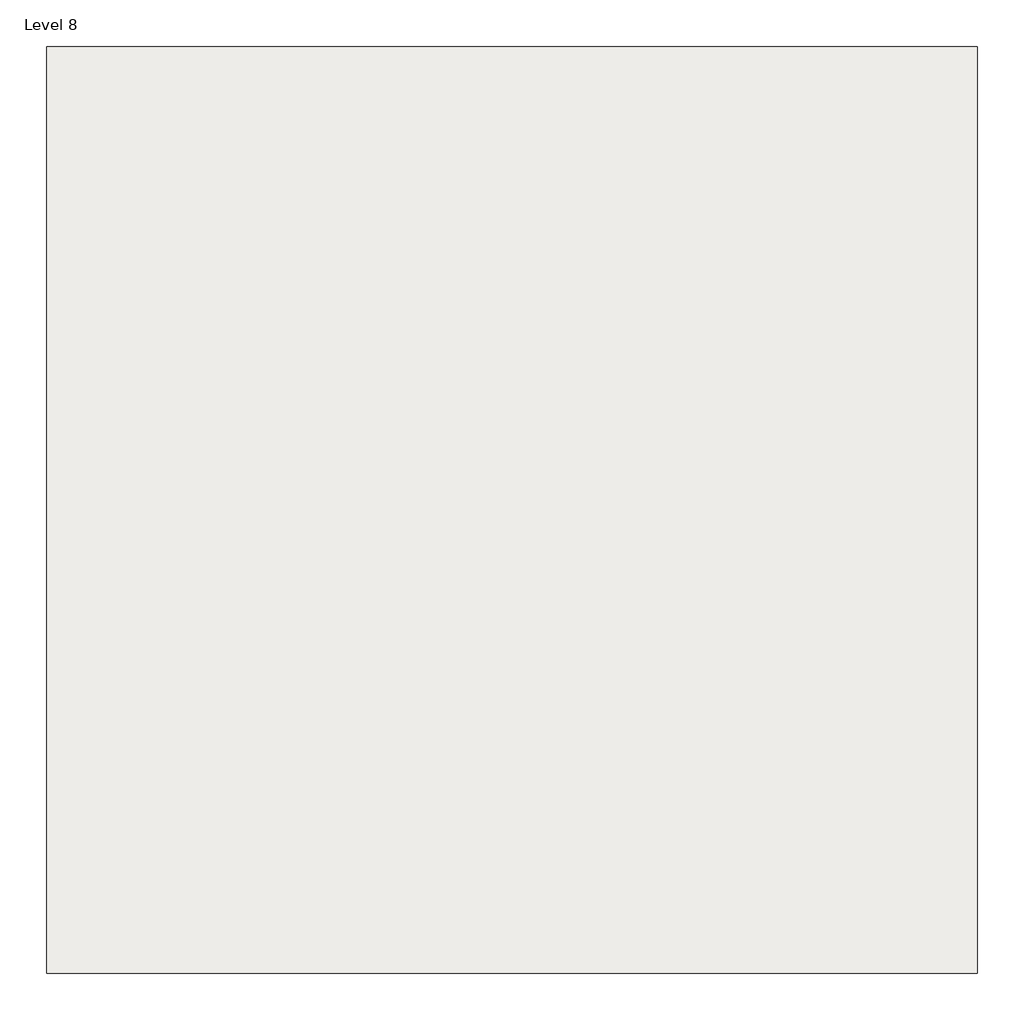
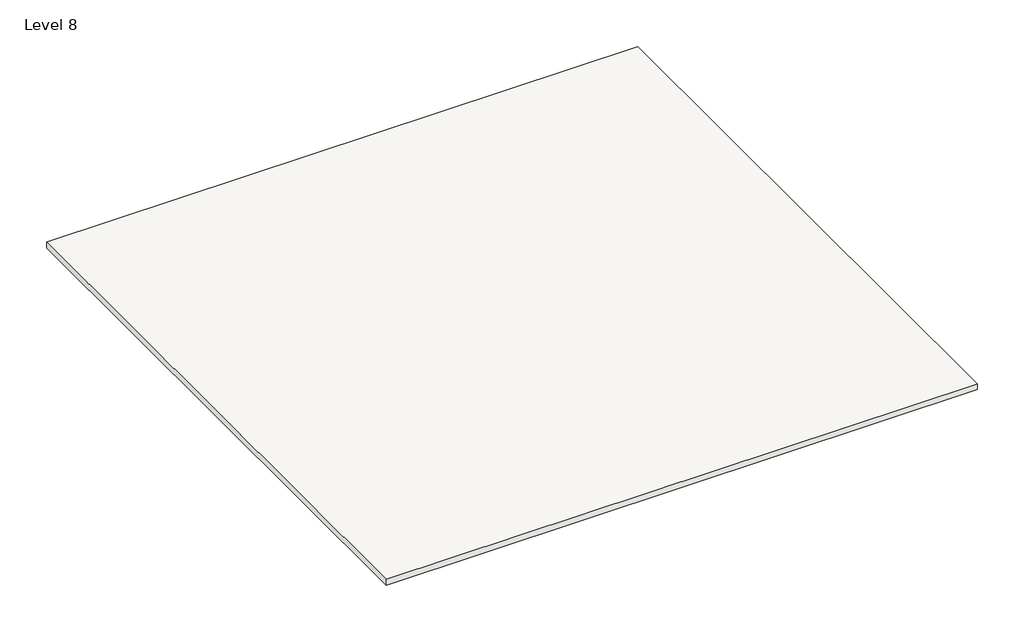
# One storey: 1 roof.
"""IFC4 building model written with IfcOpenShell, lengths in millimetres."""

from ifc_helpers import new_model, si_unit, frame, origin, place, context, project, spatial, polyline, outline, extrude, element, save

model = new_model("IFC4")

# Units and contexts
model_context = context("Model", 3, world=origin())
ifc_project = project(units=[si_unit("LENGTHUNIT", "METRE", prefix="MILLI")], contexts=[model_context])

# Site, building, storey
site = spatial("IfcSite", under=ifc_project)
building = spatial("IfcBuilding", under=site)
storey = spatial("IfcBuildingStorey", under=building, Name="Level 8", Elevation=12877.8)

# Roof
placement = place(None, origin())
element("IfcRoof", 1, ObjectType="Generic - 9\"", at=placement, inside=storey, context=model_context, shape_type="SweptSolid", body=[
    extrude(outline(polyline([(-8934.7629849, 17755.0995758), (12604.4370151, 17755.0995758), (12604.4370151, -3682.5004242), (-8934.7629849, -3682.5004242), (-8934.7629849, 17755.0995758)])), frame((0.0, 0.0, 12877.8), z_axis=(0.0, 0.0, 1.0), x_axis=(1.0, 0.0, 0.0)), (0.0, 0.0, 1.0), 228.6),
])

save(model, "model.ifc")

# Revit data of these elements
# Type "Generic - 9\""
#   Assembly Code = "B1020"
#   Layers, outside or top first: 0' - 9" no material (function 1)
# Element 1 (IfcRoof, "Generic - 9\"")
#   built-in parameter 1001705 = 43 (stored number, unit not read)
#   built-in parameter 1001710 = 33615
#   Phase Created = New Construction
#   Materials on its faces: "Default Roof"
# Materials
#   "Default Roof": colour RGB 88 101 114, transparency 0
